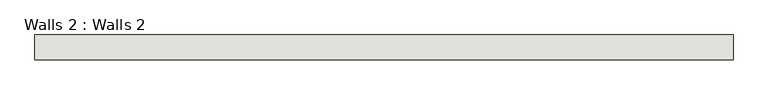
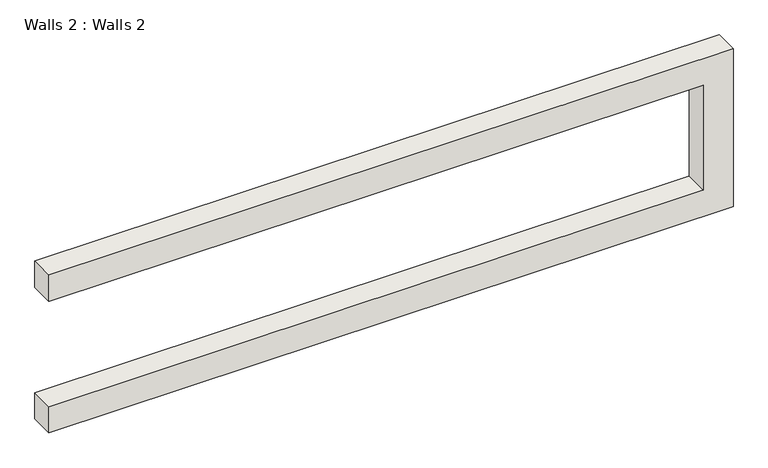
"""IFC4 building model written with IfcOpenShell, lengths in millimetres: wall geometry, Walls 2 : Walls 2."""

from ifc_helpers import new_model, si_unit, frame, origin, place, context, project, spatial, polyline, outline, extrude, source, transform, mapped, element, save


def walls_2_walls_2_f87d77c0(model_context):
    return source(origin(), model_context, "Body", "SweptSolid", [
        extrude(outline(polyline([(3505.2, -8270.822521), (2895.6, -8270.822521), (2895.6, 6711.977479), (6553.2, 6711.977479), (6553.2, -8270.822521), (5943.6, -8270.822521), (5943.6, 6054.777479), (3505.2, 6054.777479), (3505.2, -8270.822521)])), frame((0.0, -16386.6899474, 0.0), z_axis=(0.0, 1.0, 0.0), x_axis=(0.0, 0.0, 1.0)), (0.0, 0.0, 1.0), 531.1431881),
    ])


if __name__ == "__main__":
    model = new_model("IFC4")
    model_context = context("Model", 3, world=origin())
    ifc_project = project(units=[si_unit("LENGTHUNIT", "METRE", prefix="MILLI")], contexts=[model_context])
    site = spatial("IfcSite", under=ifc_project)
    building = spatial("IfcBuilding", under=site)
    placement = place(None, origin())
    walls_2_walls_2_shape = walls_2_walls_2_f87d77c0(model_context)
    element("IfcWall", 1, ObjectType="Walls 2 : Walls 2", at=placement, inside=building, context=model_context, shape_type="MappedRepresentation", body=[
        mapped(walls_2_walls_2_shape, transform((0.0, 0.0, 0.0), x_axis=(1.0, 0.0, 0.0), y_axis=(0.0, 1.0, 0.0), z_axis=(0.0, 0.0, 1.0))),
    ])
    save(model, "model.ifc")

# Revit data of these elements
# Element 1 (IfcWall, "Walls 2 : Walls 2")
#   Materials on its faces: "CREAM WALL"
# Materials
#   "CREAM WALL": colour RGB 255 255 187, transparency 0, Cost = 0
